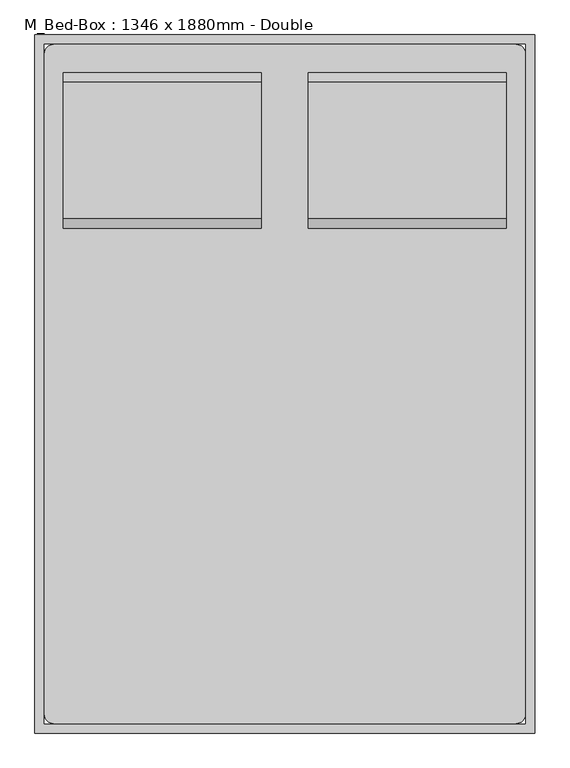
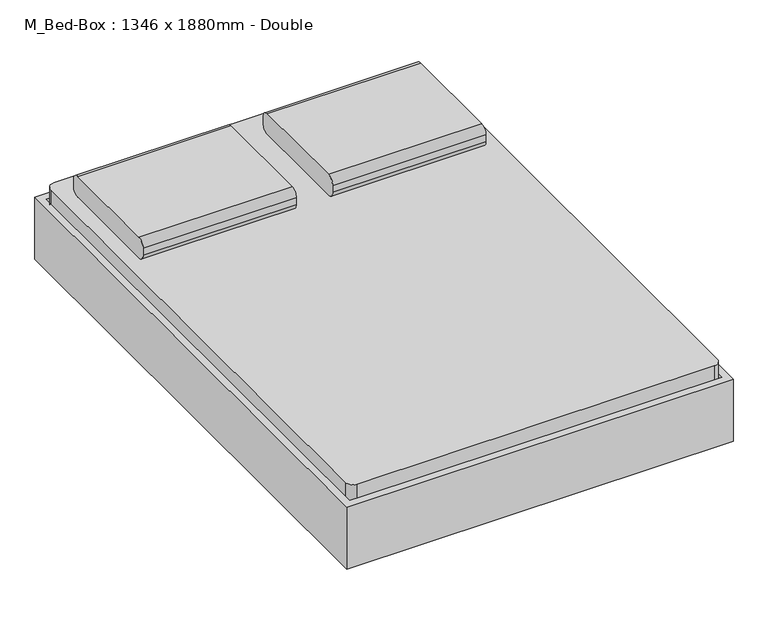
"""IFC4 building model written with IfcOpenShell, lengths in millimetres: furniture geometry, M_Bed-Box : 1346 x 1880mm - Double."""

from ifc_helpers import new_model, si_unit, point, frame, frame_2d, origin, place, context, project, spatial, polyline, circle_curve, trimmed, segment, composite_curve, outline, extrude, source, transform, mapped, element, save
from ifc_brep_helpers import plane_surface, cylinder_surface, revolved_surface, advanced_brep


def m_bed_box_1346_x_1880mm_double_b32eb57e(model_context):
    return source(origin(), model_context, "Body", "SolidModel", [
        extrude(outline(composite_curve([segment(polyline([(578.5704918, 406.4), (210.2704918, 406.4)]), True, "CONTINUOUS"), segment(trimmed(circle_curve(frame_2d((210.2704918, 431.8)), 25.4), [point((210.2704918, 406.4))], [point((184.8704918, 431.8))], False, "CARTESIAN"), True, "CONTINUOUS"), segment(polyline([(184.8704918, 431.8), (184.8704918, 457.2)]), True, "CONTINUOUS"), segment(trimmed(circle_curve(frame_2d((210.2704918, 457.2)), 25.4), [point((184.8704918, 457.2))], [point((210.2704918, 482.6))], False, "CARTESIAN"), True, "CONTINUOUS"), segment(polyline([(210.2704918, 482.6), (578.5704918, 482.6)]), True, "CONTINUOUS"), segment(trimmed(circle_curve(frame_2d((578.5704918, 457.2)), 25.4), [point((578.5704918, 482.6))], [point((603.9704918, 457.2))], False, "CARTESIAN"), True, "CONTINUOUS"), segment(polyline([(603.9704918, 457.2), (603.9704918, 431.8)]), True, "CONTINUOUS"), segment(trimmed(circle_curve(frame_2d((578.5704918, 431.8)), 25.4), [point((603.9704918, 431.8))], [point((578.5704918, 406.4))], False, "CARTESIAN"), True, "CONTINUOUS")], self_intersect=False)), frame((402.652459, 0.0, 0.0), z_axis=(1.0, 0.0, 0.0), x_axis=(0.0, 1.0, 0.0)), (0.0, 0.0, 1.0), 533.3),
        extrude(outline(composite_curve([segment(polyline([(578.5704918, 406.4), (210.2704918, 406.4)]), True, "CONTINUOUS"), segment(trimmed(circle_curve(frame_2d((210.2704918, 431.8)), 25.4), [point((210.2704918, 406.4))], [point((184.8704918, 431.8))], False, "CARTESIAN"), True, "CONTINUOUS"), segment(polyline([(184.8704918, 431.8), (184.8704918, 457.2)]), True, "CONTINUOUS"), segment(trimmed(circle_curve(frame_2d((210.2704918, 457.2)), 25.4), [point((184.8704918, 457.2))], [point((210.2704918, 482.6))], False, "CARTESIAN"), True, "CONTINUOUS"), segment(polyline([(210.2704918, 482.6), (578.5704918, 482.6)]), True, "CONTINUOUS"), segment(trimmed(circle_curve(frame_2d((578.5704918, 457.2)), 25.4), [point((578.5704918, 482.6))], [point((603.9704918, 457.2))], False, "CARTESIAN"), True, "CONTINUOUS"), segment(polyline([(603.9704918, 457.2), (603.9704918, 431.8)]), True, "CONTINUOUS"), segment(trimmed(circle_curve(frame_2d((578.5704918, 431.8)), 25.4), [point((603.9704918, 431.8))], [point((578.5704918, 406.4))], False, "CARTESIAN"), True, "CONTINUOUS")], self_intersect=False)), frame((-257.647541, 0.0, 0.0), z_axis=(1.0, 0.0, 0.0), x_axis=(0.0, 1.0, 0.0)), (0.0, 0.0, 1.0), 533.3),
        advanced_brep(
        [(-308.1231784, 451.5704918, 177.8), (-308.1231784, 375.3704918, 177.8), (-308.1231784, 375.3704918, 196.85), (-308.1231784, 451.5704918, 196.85), (-257.3231784, 451.5704918, 177.8), (-257.3231784, 375.3704918, 177.8), (-245.1869899, 375.3704918, 196.85), (-245.1869899, 451.5704918, 196.85), (-181.2523099, 451.5704918, 14.6654962), (-181.2523099, 375.3704918, 14.6654962), (-163.9871466, 375.3704918, 22.716374), (-163.9871466, 451.5704918, 22.716374), (-158.2320921, 375.3704918, 0.0), (-158.2320921, 451.5704918, 0.0), (-158.2320921, 375.3704918, 19.05), (-158.2320921, 451.5704918, 19.05), (-79.6195862, 451.5704918, 0.0), (-79.6195862, 375.3704918, 0.0), (-79.6195862, 375.3704918, 19.05), (-79.6195862, 451.5704918, 19.05), (-66.9195862, 375.3704918, 3.4029547), (-66.9195862, 451.5704918, 3.4029547), (-76.4445862, 375.3704918, 19.9007387), (-76.4445862, 451.5704918, 19.9007387), (-6.822541, 451.5704918, 38.1), (-6.822541, 375.3704918, 38.1), (-11.9269731, 375.3704918, 57.15), (-11.9269731, 451.5704918, 57.15), (685.4518216, 451.5704918, 38.1), (685.4518216, 375.3704918, 38.1), (690.5562537, 375.3704918, 57.15), (690.5562537, 451.5704918, 57.15), (745.5488669, 451.5704918, 3.4029547), (745.5488669, 375.3704918, 3.4029547), (755.0738669, 375.3704918, 19.9007387), (755.0738669, 451.5704918, 19.9007387), (758.2488669, 375.3704918, 0.0), (758.2488669, 451.5704918, 0.0), (758.2488669, 375.3704918, 19.05), (758.2488669, 451.5704918, 19.05), (836.8613728, 451.5704918, 0.0), (836.8613728, 375.3704918, 0.0), (836.8613728, 375.3704918, 19.05), (836.8613728, 451.5704918, 19.05), (859.8815906, 375.3704918, 14.6654962), (859.8815906, 451.5704918, 14.6654962), (842.6164272, 375.3704918, 22.716374), (842.6164272, 451.5704918, 22.716374), (935.952459, 451.5704918, 177.8), (935.952459, 375.3704918, 177.8), (923.8162705, 375.3704918, 196.85), (923.8162705, 451.5704918, 196.85), (986.752459, 451.5704918, 177.8), (986.752459, 451.5704918, 196.85), (986.752459, 375.3704918, 196.85), (986.752459, 375.3704918, 177.8)],
        [
            (0, 1),
            (1, 2),
            (2, 3),
            (3, 0),
            (0, 4),
            (4, 5),
            (5, 1),
            (5, 6),
            (6, 2),
            (6, 7),
            (7, 3),
            (7, 4),
            (4, 8),
            (8, 9),
            (9, 5),
            (9, 10),
            (10, 6),
            (10, 11),
            (11, 7),
            (11, 8),
            (12, 9, circle_curve(frame((-158.2320921, 375.3704918, 25.4), z_axis=(0.0, 1.0, 0.0), x_axis=(-0.906307787036649, 0.0, -0.4226182617407015)), 25.4)),
            (8, 13, circle_curve(frame((-158.2320921, 451.5704918, 25.4), z_axis=(0.0, -1.0, 0.0), x_axis=(-0.906307787036649, 0.0, -0.4226182617407015)), 25.4)),
            (13, 12),
            (14, 10, circle_curve(frame((-158.2320921, 375.3704918, 25.4), z_axis=(0.0, 1.0, 0.0), x_axis=(-0.906307787036649, 0.0, -0.4226182617407015)), 6.35)),
            (12, 14),
            (15, 11, circle_curve(frame((-158.2320921, 451.5704918, 25.4), z_axis=(0.0, 1.0, 0.0), x_axis=(-0.906307787036649, 0.0, -0.4226182617407015)), 6.35)),
            (14, 15),
            (15, 13),
            (13, 16),
            (16, 17),
            (17, 12),
            (17, 18),
            (18, 14),
            (18, 19),
            (19, 15),
            (19, 16),
            (20, 17, circle_curve(frame((-79.6195862, 375.3704918, 25.4), z_axis=(0.0, 1.0, 0.0), x_axis=(0.0, 0.0, -1.0)), 25.4)),
            (16, 21, circle_curve(frame((-79.6195862, 451.5704918, 25.4), z_axis=(0.0, -1.0, 0.0), x_axis=(0.0, 0.0, -1.0)), 25.4)),
            (21, 20),
            (22, 18, circle_curve(frame((-79.6195862, 375.3704918, 25.4), z_axis=(0.0, 1.0, 0.0), x_axis=(0.0, 0.0, -1.0)), 6.35)),
            (20, 22),
            (23, 19, circle_curve(frame((-79.6195862, 451.5704918, 25.4), z_axis=(0.0, 1.0, 0.0), x_axis=(0.0, 0.0, -1.0)), 6.35)),
            (22, 23),
            (23, 21),
            (21, 24),
            (24, 25),
            (25, 20),
            (25, 26),
            (26, 22),
            (26, 27),
            (27, 23),
            (27, 24),
            (24, 28),
            (28, 29),
            (29, 25),
            (29, 30),
            (30, 26),
            (30, 31),
            (31, 27),
            (31, 28),
            (28, 32),
            (32, 33),
            (33, 29),
            (33, 34),
            (34, 30),
            (34, 35),
            (35, 31),
            (35, 32),
            (36, 33, circle_curve(frame((758.2488669, 375.3704918, 25.4), z_axis=(0.0, 1.0, 0.0), x_axis=(-0.5000000000000463, 0.0, -0.8660254037844118)), 25.4)),
            (32, 37, circle_curve(frame((758.2488669, 451.5704918, 25.4), z_axis=(0.0, -1.0, 0.0), x_axis=(-0.5000000000000463, 0.0, -0.8660254037844118)), 25.4)),
            (37, 36),
            (38, 34, circle_curve(frame((758.2488669, 375.3704918, 25.4), z_axis=(0.0, 1.0, 0.0), x_axis=(-0.5000000000000463, 0.0, -0.8660254037844118)), 6.35)),
            (36, 38),
            (39, 35, circle_curve(frame((758.2488669, 451.5704918, 25.4), z_axis=(0.0, 1.0, 0.0), x_axis=(-0.5000000000000463, 0.0, -0.8660254037844118)), 6.35)),
            (38, 39),
            (39, 37),
            (37, 40),
            (40, 41),
            (41, 36),
            (41, 42),
            (42, 38),
            (42, 43),
            (43, 39),
            (43, 40),
            (44, 41, circle_curve(frame((836.8613728, 375.3704918, 25.4), z_axis=(0.0, 1.0, 0.0), x_axis=(0.0, 0.0, -1.0)), 25.4)),
            (40, 45, circle_curve(frame((836.8613728, 451.5704918, 25.4), z_axis=(0.0, -1.0, 0.0), x_axis=(0.0, 0.0, -1.0)), 25.4)),
            (45, 44),
            (46, 42, circle_curve(frame((836.8613728, 375.3704918, 25.4), z_axis=(0.0, 1.0, 0.0), x_axis=(0.0, 0.0, -1.0)), 6.35)),
            (44, 46),
            (47, 43, circle_curve(frame((836.8613728, 451.5704918, 25.4), z_axis=(0.0, 1.0, 0.0), x_axis=(0.0, 0.0, -1.0)), 6.35)),
            (46, 47),
            (47, 45),
            (45, 48),
            (48, 49),
            (49, 44),
            (49, 50),
            (50, 46),
            (50, 51),
            (51, 47),
            (51, 48),
            (52, 53),
            (53, 54),
            (54, 55),
            (55, 52),
            (48, 52),
            (55, 49),
            (54, 50),
            (53, 51),
        ],
        [
            plane_surface(frame((-308.1231784, 705.5704918, -152.9490627), z_axis=(-1.0, 0.0, 0.0), x_axis=(0.0, 1.0, 0.0))),
            plane_surface(frame((-308.1231784, 451.5704918, 177.8), z_axis=(0.0, 0.0, -1.0), x_axis=(1.0, 0.0, 0.0))),
            plane_surface(frame((-308.1231784, 375.3704918, 177.8), z_axis=(0.0, -1.0, 0.0), x_axis=(1.0, 0.0, 0.0))),
            plane_surface(frame((-308.1231784, 375.3704918, 196.85), z_axis=(0.0, 0.0, 1.0), x_axis=(1.0, 0.0, 0.0))),
            plane_surface(frame((-308.1231784, 451.5704918, 196.85), z_axis=(0.0, 1.0, 0.0), x_axis=(1.0, 0.0, 0.0))),
            plane_surface(frame((-257.3231784, 451.5704918, 177.8), z_axis=(-0.9063077870366486, 0.0, -0.4226182617407026), x_axis=(0.4226182617407026, 0.0, -0.9063077870366486))),
            plane_surface(frame((-257.3231784, 375.3704918, 177.8), z_axis=(0.0, -1.0000000000000002, 0.0), x_axis=(0.4226182617407026, 0.0, -0.9063077870366486))),
            plane_surface(frame((-245.1869899, 375.3704918, 196.85), z_axis=(0.9063077870366487, 0.0, 0.4226182617407023), x_axis=(0.4226182617407023, 0.0, -0.9063077870366487))),
            plane_surface(frame((-245.1869899, 451.5704918, 196.85), z_axis=(0.0, 1.0, 0.0), x_axis=(0.4226182617407027, 0.0, -0.9063077870366485))),
            cylinder_surface(frame((-158.2320921, 705.5704918, 25.4), z_axis=(0.0, -1.0, 0.0), x_axis=(-0.906307787036649, 0.0, -0.4226182617407015)), 25.4),
            plane_surface(frame((-158.2320921, 375.3704918, 25.4), z_axis=(0.0, -1.0, 0.0), x_axis=(-0.906307787036649, 0.0, -0.4226182617407015))),
            revolved_surface(polyline([(-163.9871465476827, 375.3704918, 22.716374037946544), (-163.9871465476827, 451.5704918, 22.716374037946544)]), (-158.2320921, 705.5704918, 25.4), (0.0, -1.0, 0.0)),
            plane_surface(frame((-158.2320921, 451.5704918, 25.4), z_axis=(0.0, 1.0, 0.0), x_axis=(-0.906307787036649, 0.0, -0.4226182617407015))),
            plane_surface(frame((-158.2320921, 451.5704918, 0.0), z_axis=(0.0, 0.0, -1.0), x_axis=(1.0, 0.0, 0.0))),
            plane_surface(frame((-158.2320921, 375.3704918, 0.0), z_axis=(0.0, -1.0, 0.0), x_axis=(1.0, 0.0, 0.0))),
            plane_surface(frame((-158.2320921, 375.3704918, 19.05), z_axis=(0.0, 0.0, 1.0), x_axis=(1.0, 0.0, 0.0))),
            plane_surface(frame((-158.2320921, 451.5704918, 19.05), z_axis=(0.0, 1.0, 0.0), x_axis=(1.0, 0.0, 0.0))),
            cylinder_surface(frame((-79.6195862, 705.5704918, 25.4), z_axis=(0.0, -1.0, 0.0), x_axis=(0.0, 0.0, -1.0)), 25.4),
            plane_surface(frame((-79.6195862, 375.3704918, 25.4), z_axis=(0.0, -1.0, 0.0), x_axis=(0.0, 0.0, -1.0))),
            revolved_surface(polyline([(-79.6195862, 375.3704918, 19.049999999999997), (-79.6195862, 451.5704918, 19.049999999999997)]), (-79.6195862, 705.5704918, 25.4), (0.0, -1.0, 0.0)),
            plane_surface(frame((-79.6195862, 451.5704918, 25.4), z_axis=(0.0, 1.0, 0.0), x_axis=(0.0, 0.0, -1.0))),
            plane_surface(frame((-66.9195862, 451.5704918, 3.4029547), z_axis=(0.4999999999998744, 0.0, -0.8660254037845112), x_axis=(0.8660254037845112, 0.0, 0.4999999999998744))),
            plane_surface(frame((-66.9195862, 375.3704918, 3.4029547), z_axis=(0.0, -1.0000000000000002, 0.0), x_axis=(0.8660254037845112, 0.0, 0.4999999999998745))),
            plane_surface(frame((-76.4445862, 375.3704918, 19.9007387), z_axis=(-0.4999999999998741, 0.0, 0.8660254037845113), x_axis=(0.8660254037845113, 0.0, 0.4999999999998741))),
            plane_surface(frame((-76.4445862, 451.5704918, 19.9007387), z_axis=(0.0, 1.0, 0.0), x_axis=(0.866025403784511, 0.0, 0.49999999999987477))),
            plane_surface(frame((-6.822541, 451.5704918, 38.1), z_axis=(0.0, 0.0, -1.0), x_axis=(1.0, 0.0, 0.0))),
            plane_surface(frame((-6.822541, 375.3704918, 38.1), z_axis=(0.0, -1.0, 0.0), x_axis=(1.0, 0.0, 0.0))),
            plane_surface(frame((-11.9269731, 375.3704918, 57.15), z_axis=(0.0, 0.0, 1.0), x_axis=(1.0, 0.0, 0.0))),
            plane_surface(frame((-11.9269731, 451.5704918, 57.15), z_axis=(0.0, 1.0, 0.0), x_axis=(1.0, 0.0, 0.0))),
            plane_surface(frame((685.4518216, 451.5704918, 38.1), z_axis=(-0.5000000000000494, 0.0, -0.8660254037844102), x_axis=(0.8660254037844102, 0.0, -0.5000000000000494))),
            plane_surface(frame((685.4518216, 375.3704918, 38.1), z_axis=(0.0, -1.0, 0.0), x_axis=(0.8660254037844112, 0.0, -0.5000000000000476))),
            plane_surface(frame((690.5562537, 375.3704918, 57.15), z_axis=(0.5000000000000488, 0.0, 0.8660254037844105), x_axis=(0.8660254037844105, 0.0, -0.5000000000000488))),
            plane_surface(frame((690.5562537, 451.5704918, 57.15), z_axis=(0.0, 1.0, 0.0), x_axis=(0.8660254037844106, 0.0, -0.5000000000000485))),
            cylinder_surface(frame((758.2488669, 705.5704918, 25.4), z_axis=(0.0, -1.0, 0.0), x_axis=(-0.5000000000000463, 0.0, -0.8660254037844118)), 25.4),
            plane_surface(frame((758.2488669, 375.3704918, 25.4), z_axis=(0.0, -1.0000000000000002, 0.0), x_axis=(-0.5000000000000464, 0.0, -0.866025403784412))),
            revolved_surface(polyline([(755.0738668999998, 375.3704918, 19.90073868596898), (755.0738668999998, 451.5704918, 19.90073868596898)]), (758.2488669, 705.5704918, 25.4), (0.0, -1.0, 0.0)),
            plane_surface(frame((758.2488669, 451.5704918, 25.4), z_axis=(0.0, 1.0000000000000002, 0.0), x_axis=(-0.5000000000000464, 0.0, -0.866025403784412))),
            plane_surface(frame((758.2488669, 451.5704918, 0.0), z_axis=(0.0, 0.0, -1.0), x_axis=(1.0, 0.0, 0.0))),
            plane_surface(frame((758.2488669, 375.3704918, 0.0), z_axis=(0.0, -1.0, 0.0), x_axis=(1.0, 0.0, 0.0))),
            plane_surface(frame((758.2488669, 375.3704918, 19.05), z_axis=(0.0, 0.0, 1.0), x_axis=(1.0, 0.0, 0.0))),
            plane_surface(frame((758.2488669, 451.5704918, 19.05), z_axis=(0.0, 1.0, 0.0), x_axis=(1.0, 0.0, 0.0))),
            cylinder_surface(frame((836.8613728, 705.5704918, 25.4), z_axis=(0.0, -1.0, 0.0), x_axis=(0.0, 0.0, -1.0)), 25.4),
            plane_surface(frame((836.8613728, 375.3704918, 25.4), z_axis=(0.0, -1.0, 0.0), x_axis=(0.0, 0.0, -1.0))),
            revolved_surface(polyline([(836.8613728, 375.3704918, 19.049999999999997), (836.8613728, 451.5704918, 19.049999999999997)]), (836.8613728, 705.5704918, 25.4), (0.0, -1.0, 0.0)),
            plane_surface(frame((836.8613728, 451.5704918, 25.4), z_axis=(0.0, 1.0, 0.0), x_axis=(0.0, 0.0, -1.0))),
            plane_surface(frame((859.8815906, 451.5704918, 14.6654962), z_axis=(0.90630778703668, 0.0, -0.422618261740635), x_axis=(0.422618261740635, 0.0, 0.90630778703668))),
            plane_surface(frame((859.8815906, 375.3704918, 14.6654962), z_axis=(0.0, -1.0000000000000002, 0.0), x_axis=(0.4226182617406349, 0.0, 0.9063077870366801))),
            plane_surface(frame((842.6164272, 375.3704918, 22.716374), z_axis=(-0.9063077870366805, 0.0, 0.4226182617406341), x_axis=(0.4226182617406341, 0.0, 0.9063077870366805))),
            plane_surface(frame((842.6164272, 451.5704918, 22.716374), z_axis=(0.0, 1.0, 0.0), x_axis=(0.42261826174063455, 0.0, 0.9063077870366802))),
            plane_surface(frame((986.752459, 705.5704918, -152.9490627), z_axis=(1.0, 0.0, 0.0), x_axis=(0.0, 1.0, 0.0))),
            plane_surface(frame((935.952459, 451.5704918, 177.8), z_axis=(0.0, 0.0, -1.0), x_axis=(1.0, 0.0, 0.0))),
            plane_surface(frame((935.952459, 375.3704918, 177.8), z_axis=(0.0, -1.0, 0.0), x_axis=(1.0, 0.0, 0.0))),
            plane_surface(frame((923.8162705, 375.3704918, 196.85), z_axis=(0.0, 0.0, 1.0), x_axis=(1.0, 0.0, 0.0))),
            plane_surface(frame((923.8162705, 451.5704918, 196.85), z_axis=(0.0, 1.0, 0.0), x_axis=(1.0, 0.0, 0.0))),
        ],
        [
            (0, [[1, 2, 3, 4]]),
            (1, [[-1, 5, 6, 7]]),
            (2, [[-2, -7, 8, 9]]),
            (3, [[-3, -9, 10, 11]]),
            (4, [[-4, -11, 12, -5]]),
            (5, [[-6, 13, 14, 15]]),
            (6, [[-8, -15, 16, 17]]),
            (7, [[-10, -17, 18, 19]]),
            (8, [[-12, -19, 20, -13]]),
            (9, [[21, -14, 22, 23]]),
            (10, [[24, -16, -21, 25]]),
            (11, [[26, -18, -24, 27]]),
            (12, [[-22, -20, -26, 28]]),
            (13, [[-23, 29, 30, 31]]),
            (14, [[-25, -31, 32, 33]]),
            (15, [[-27, -33, 34, 35]]),
            (16, [[-28, -35, 36, -29]]),
            (17, [[37, -30, 38, 39]]),
            (18, [[40, -32, -37, 41]]),
            (19, [[42, -34, -40, 43]]),
            (20, [[-38, -36, -42, 44]]),
            (21, [[-39, 45, 46, 47]]),
            (22, [[-41, -47, 48, 49]]),
            (23, [[-43, -49, 50, 51]]),
            (24, [[-44, -51, 52, -45]]),
            (25, [[-46, 53, 54, 55]]),
            (26, [[-48, -55, 56, 57]]),
            (27, [[-50, -57, 58, 59]]),
            (28, [[-52, -59, 60, -53]]),
            (29, [[-54, 61, 62, 63]]),
            (30, [[-56, -63, 64, 65]]),
            (31, [[-58, -65, 66, 67]]),
            (32, [[-60, -67, 68, -61]]),
            (33, [[69, -62, 70, 71]]),
            (34, [[72, -64, -69, 73]]),
            (35, [[74, -66, -72, 75]]),
            (36, [[-70, -68, -74, 76]]),
            (37, [[-71, 77, 78, 79]]),
            (38, [[-73, -79, 80, 81]]),
            (39, [[-75, -81, 82, 83]]),
            (40, [[-76, -83, 84, -77]]),
            (41, [[85, -78, 86, 87]]),
            (42, [[88, -80, -85, 89]]),
            (43, [[90, -82, -88, 91]]),
            (44, [[-86, -84, -90, 92]]),
            (45, [[-87, 93, 94, 95]]),
            (46, [[-89, -95, 96, 97]]),
            (47, [[-91, -97, 98, 99]]),
            (48, [[-92, -99, 100, -93]]),
            (49, [[101, 102, 103, 104]]),
            (50, [[-94, 105, -104, 106]]),
            (51, [[-96, -106, -103, 107]]),
            (52, [[-98, -107, -102, 108]]),
            (53, [[-100, -108, -101, -105]]),
        ],
    ),
        extrude(outline(composite_curve([segment(polyline([(-283.047541, 680.1704918), (961.352459, 680.1704918)]), True, "CONTINUOUS"), segment(trimmed(circle_curve(frame_2d((961.352459, 654.7704918)), 25.4), [point((961.352459, 680.1704918))], [point((986.752459, 654.7704918))], False, "CARTESIAN"), True, "CONTINUOUS"), segment(polyline([(986.752459, 654.7704918), (986.752459, -1123.6295082)]), True, "CONTINUOUS"), segment(trimmed(circle_curve(frame_2d((961.352459, -1123.6295082)), 25.4), [point((986.752459, -1123.6295082))], [point((961.352459, -1149.0295082))], False, "CARTESIAN"), True, "CONTINUOUS"), segment(polyline([(961.352459, -1149.0295082), (-283.047541, -1149.0295082)]), True, "CONTINUOUS"), segment(trimmed(circle_curve(frame_2d((-283.047541, -1123.6295082)), 25.4), [point((-283.047541, -1149.0295082))], [point((-308.447541, -1123.6295082))], False, "CARTESIAN"), True, "CONTINUOUS"), segment(polyline([(-308.447541, -1123.6295082), (-308.447541, 654.7704918)]), True, "CONTINUOUS"), segment(trimmed(circle_curve(frame_2d((-283.047541, 654.7704918)), 25.4), [point((-308.447541, 654.7704918))], [point((-283.047541, 680.1704918))], False, "CARTESIAN"), True, "CONTINUOUS")], self_intersect=False)), frame((0.0, 0.0, 203.2), z_axis=(0.0, 0.0, 1.0), x_axis=(1.0, 0.0, 0.0)), (0.0, 0.0, 1.0), 203.2),
        advanced_brep(
        [(-308.447541, -869.6295082, 196.85), (-308.447541, -869.6295082, 177.8), (-308.447541, -945.8295082, 177.8), (-308.447541, -945.8295082, 196.85), (-245.5113525, -869.6295082, 196.85), (-257.647541, -869.6295082, 177.8), (-257.647541, -945.8295082, 177.8), (-245.5113525, -945.8295082, 196.85), (-164.3115092, -869.6295082, 22.716374), (-181.5766725, -869.6295082, 14.6654962), (-181.5766725, -945.8295082, 14.6654962), (-164.3115092, -945.8295082, 22.716374), (-158.5564547, -869.6295082, 0.0), (-158.5564547, -869.6295082, 19.05), (-158.5564547, -945.8295082, 0.0), (-158.5564547, -945.8295082, 19.05), (-79.9439489, -869.6295082, 19.05), (-79.9439489, -869.6295082, 0.0), (-79.9439489, -945.8295082, 0.0), (-79.9439489, -945.8295082, 19.05), (-67.2439489, -869.6295082, 3.4029547), (-76.7689489, -869.6295082, 19.9007387), (-67.2439489, -945.8295082, 3.4029547), (-76.7689489, -945.8295082, 19.9007387), (-12.2513357, -869.6295082, 57.15), (-7.1469036, -869.6295082, 38.1), (-7.1469036, -945.8295082, 38.1), (-12.2513357, -945.8295082, 57.15), (690.5562537, -869.6295082, 57.15), (685.4518216, -869.6295082, 38.1), (685.4518216, -945.8295082, 38.1), (690.5562537, -945.8295082, 57.15), (755.0738669, -869.6295082, 19.9007387), (745.5488669, -869.6295082, 3.4029547), (745.5488669, -945.8295082, 3.4029547), (755.0738669, -945.8295082, 19.9007387), (758.2488669, -869.6295082, 0.0), (758.2488669, -869.6295082, 19.05), (758.2488669, -945.8295082, 0.0), (758.2488669, -945.8295082, 19.05), (836.8613728, -869.6295082, 19.05), (836.8613728, -869.6295082, 0.0), (836.8613728, -945.8295082, 0.0), (836.8613728, -945.8295082, 19.05), (859.8815906, -869.6295082, 14.6654962), (842.6164272, -869.6295082, 22.716374), (859.8815906, -945.8295082, 14.6654962), (842.6164272, -945.8295082, 22.716374), (923.8162705, -869.6295082, 196.85), (935.952459, -869.6295082, 177.8), (935.952459, -945.8295082, 177.8), (923.8162705, -945.8295082, 196.85), (986.752459, -869.6295082, 196.85), (986.752459, -945.8295082, 196.85), (986.752459, -945.8295082, 177.8), (986.752459, -869.6295082, 177.8)],
        [
            (0, 1),
            (1, 2),
            (2, 3),
            (3, 0),
            (0, 4),
            (4, 5),
            (5, 1),
            (5, 6),
            (6, 2),
            (6, 7),
            (7, 3),
            (7, 4),
            (4, 8),
            (8, 9),
            (9, 5),
            (9, 10),
            (10, 6),
            (10, 11),
            (11, 7),
            (11, 8),
            (12, 9, circle_curve(frame((-158.5564547, -869.6295082, 25.4), z_axis=(0.0, 1.0, 0.0), x_axis=(-0.9063077870366625, 0.0, -0.4226182617406725)), 25.4)),
            (8, 13, circle_curve(frame((-158.5564547, -869.6295082, 25.4), z_axis=(0.0, -1.0, 0.0), x_axis=(-0.9063077870366625, 0.0, -0.4226182617406725)), 6.35)),
            (13, 12),
            (14, 10, circle_curve(frame((-158.5564547, -945.8295082, 25.4), z_axis=(0.0, 1.0, 0.0), x_axis=(-0.9063077870366625, 0.0, -0.4226182617406725)), 25.4)),
            (12, 14),
            (15, 11, circle_curve(frame((-158.5564547, -945.8295082, 25.4), z_axis=(0.0, 1.0, 0.0), x_axis=(-0.9063077870366625, 0.0, -0.4226182617406725)), 6.35)),
            (14, 15),
            (15, 13),
            (13, 16),
            (16, 17),
            (17, 12),
            (17, 18),
            (18, 14),
            (18, 19),
            (19, 15),
            (19, 16),
            (20, 17, circle_curve(frame((-79.9439489, -869.6295082, 25.4), z_axis=(0.0, 1.0, 0.0), x_axis=(0.0, 0.0, -1.0)), 25.4)),
            (16, 21, circle_curve(frame((-79.9439489, -869.6295082, 25.4), z_axis=(0.0, -1.0, 0.0), x_axis=(0.0, 0.0, -1.0)), 6.35)),
            (21, 20),
            (22, 18, circle_curve(frame((-79.9439489, -945.8295082, 25.4), z_axis=(0.0, 1.0, 0.0), x_axis=(0.0, 0.0, -1.0)), 25.4)),
            (20, 22),
            (23, 19, circle_curve(frame((-79.9439489, -945.8295082, 25.4), z_axis=(0.0, 1.0, 0.0), x_axis=(0.0, 0.0, -1.0)), 6.35)),
            (22, 23),
            (23, 21),
            (21, 24),
            (24, 25),
            (25, 20),
            (25, 26),
            (26, 22),
            (26, 27),
            (27, 23),
            (27, 24),
            (24, 28),
            (28, 29),
            (29, 25),
            (29, 30),
            (30, 26),
            (30, 31),
            (31, 27),
            (31, 28),
            (28, 32),
            (32, 33),
            (33, 29),
            (33, 34),
            (34, 30),
            (34, 35),
            (35, 31),
            (35, 32),
            (36, 33, circle_curve(frame((758.2488669, -869.6295082, 25.4), z_axis=(0.0, 1.0, 0.0), x_axis=(-0.5000000000000528, 0.0, -0.8660254037844081)), 25.4)),
            (32, 37, circle_curve(frame((758.2488669, -869.6295082, 25.4), z_axis=(0.0, -1.0, 0.0), x_axis=(-0.5000000000000528, 0.0, -0.8660254037844081)), 6.35)),
            (37, 36),
            (38, 34, circle_curve(frame((758.2488669, -945.8295082, 25.4), z_axis=(0.0, 1.0, 0.0), x_axis=(-0.5000000000000528, 0.0, -0.8660254037844081)), 25.4)),
            (36, 38),
            (39, 35, circle_curve(frame((758.2488669, -945.8295082, 25.4), z_axis=(0.0, 1.0, 0.0), x_axis=(-0.5000000000000528, 0.0, -0.8660254037844081)), 6.35)),
            (38, 39),
            (39, 37),
            (37, 40),
            (40, 41),
            (41, 36),
            (41, 42),
            (42, 38),
            (42, 43),
            (43, 39),
            (43, 40),
            (44, 41, circle_curve(frame((836.8613728, -869.6295082, 25.4), z_axis=(0.0, 1.0, 0.0), x_axis=(0.0, 0.0, -1.0)), 25.4)),
            (40, 45, circle_curve(frame((836.8613728, -869.6295082, 25.4), z_axis=(0.0, -1.0, 0.0), x_axis=(0.0, 0.0, -1.0)), 6.35)),
            (45, 44),
            (46, 42, circle_curve(frame((836.8613728, -945.8295082, 25.4), z_axis=(0.0, 1.0, 0.0), x_axis=(0.0, 0.0, -1.0)), 25.4)),
            (44, 46),
            (47, 43, circle_curve(frame((836.8613728, -945.8295082, 25.4), z_axis=(0.0, 1.0, 0.0), x_axis=(0.0, 0.0, -1.0)), 6.35)),
            (46, 47),
            (47, 45),
            (45, 48),
            (48, 49),
            (49, 44),
            (49, 50),
            (50, 46),
            (50, 51),
            (51, 47),
            (51, 48),
            (52, 53),
            (53, 54),
            (54, 55),
            (55, 52),
            (48, 52),
            (55, 49),
            (54, 50),
            (53, 51),
        ],
        [
            plane_surface(frame((-308.447541, -1174.4295082, -127.5947323), z_axis=(-1.0, 0.0, 0.0), x_axis=(0.0, 1.0, 0.0))),
            plane_surface(frame((-308.447541, -869.6295082, 196.85), z_axis=(0.0, 1.0, 0.0), x_axis=(1.0, 0.0, 0.0))),
            plane_surface(frame((-308.447541, -869.6295082, 177.8), z_axis=(0.0, 0.0, -1.0), x_axis=(1.0, 0.0, 0.0))),
            plane_surface(frame((-308.447541, -945.8295082, 177.8), z_axis=(0.0, -1.0, 0.0), x_axis=(1.0, 0.0, 0.0))),
            plane_surface(frame((-308.447541, -945.8295082, 196.85), z_axis=(0.0, 0.0, 1.0), x_axis=(1.0, 0.0, 0.0))),
            plane_surface(frame((-245.5113525, -869.6295082, 196.85), z_axis=(0.0, 1.0, 0.0), x_axis=(0.4226182617406714, 0.0, -0.906307787036663))),
            plane_surface(frame((-257.647541, -869.6295082, 177.8), z_axis=(-0.9063077870366631, 0.0, -0.42261826174067146), x_axis=(0.42261826174067146, 0.0, -0.9063077870366631))),
            plane_surface(frame((-257.647541, -945.8295082, 177.8), z_axis=(0.0, -1.0000000000000002, 0.0), x_axis=(0.4226182617406716, 0.0, -0.906307787036663))),
            plane_surface(frame((-245.5113525, -945.8295082, 196.85), z_axis=(0.906307787036663, 0.0, 0.4226182617406716), x_axis=(0.4226182617406716, 0.0, -0.906307787036663))),
            plane_surface(frame((-158.5564547, -869.6295082, 25.4), z_axis=(0.0, 1.0, 0.0), x_axis=(-0.9063077870366625, 0.0, -0.4226182617406725))),
            cylinder_surface(frame((-158.5564547, -1174.4295082, 25.4), z_axis=(0.0, -1.0, 0.0), x_axis=(-0.9063077870366625, 0.0, -0.4226182617406725)), 25.4),
            plane_surface(frame((-158.5564547, -945.8295082, 25.4), z_axis=(0.0, -1.0, 0.0), x_axis=(-0.9063077870366625, 0.0, -0.4226182617406725))),
            revolved_surface(polyline([(-164.31150914768278, -945.8295082, 22.71637403794673), (-164.31150914768278, -869.6295082, 22.71637403794673)]), (-158.5564547, -1174.4295082, 25.4), (0.0, -1.0, 0.0)),
            plane_surface(frame((-158.5564547, -869.6295082, 19.05), z_axis=(0.0, 1.0, 0.0), x_axis=(1.0, 0.0, 0.0))),
            plane_surface(frame((-158.5564547, -869.6295082, 0.0), z_axis=(0.0, 0.0, -1.0), x_axis=(1.0, 0.0, 0.0))),
            plane_surface(frame((-158.5564547, -945.8295082, 0.0), z_axis=(0.0, -1.0, 0.0), x_axis=(1.0, 0.0, 0.0))),
            plane_surface(frame((-158.5564547, -945.8295082, 19.05), z_axis=(0.0, 0.0, 1.0), x_axis=(1.0, 0.0, 0.0))),
            plane_surface(frame((-79.9439489, -869.6295082, 25.4), z_axis=(0.0, 1.0, 0.0), x_axis=(0.0, 0.0, -1.0))),
            cylinder_surface(frame((-79.9439489, -1174.4295082, 25.4), z_axis=(0.0, -1.0, 0.0), x_axis=(0.0, 0.0, -1.0)), 25.4),
            plane_surface(frame((-79.9439489, -945.8295082, 25.4), z_axis=(0.0, -1.0, 0.0), x_axis=(0.0, 0.0, -1.0))),
            revolved_surface(polyline([(-79.9439489, -945.8295082, 19.049999999999997), (-79.9439489, -869.6295082, 19.049999999999997)]), (-79.9439489, -1174.4295082, 25.4), (0.0, -1.0, 0.0)),
            plane_surface(frame((-76.7689489, -869.6295082, 19.9007387), z_axis=(0.0, 1.0000000000000002, 0.0), x_axis=(0.8660254037844788, 0.0, 0.49999999999993067))),
            plane_surface(frame((-67.2439489, -869.6295082, 3.4029547), z_axis=(0.49999999999993067, 0.0, -0.8660254037844787), x_axis=(0.8660254037844787, 0.0, 0.49999999999993067))),
            plane_surface(frame((-67.2439489, -945.8295082, 3.4029547), z_axis=(0.0, -1.0, 0.0), x_axis=(0.8660254037844782, 0.0, 0.4999999999999315))),
            plane_surface(frame((-76.7689489, -945.8295082, 19.9007387), z_axis=(-0.49999999999993044, 0.0, 0.8660254037844789), x_axis=(0.8660254037844789, 0.0, 0.49999999999993044))),
            plane_surface(frame((-12.2513357, -869.6295082, 57.15), z_axis=(0.0, 1.0, 0.0), x_axis=(1.0, 0.0, 0.0))),
            plane_surface(frame((-7.1469036, -869.6295082, 38.1), z_axis=(0.0, 0.0, -1.0), x_axis=(1.0, 0.0, 0.0))),
            plane_surface(frame((-7.1469036, -945.8295082, 38.1), z_axis=(0.0, -1.0, 0.0), x_axis=(1.0, 0.0, 0.0))),
            plane_surface(frame((-12.2513357, -945.8295082, 57.15), z_axis=(0.0, 0.0, 1.0), x_axis=(1.0, 0.0, 0.0))),
            plane_surface(frame((690.5562537, -869.6295082, 57.15), z_axis=(0.0, 1.0, 0.0), x_axis=(0.8660254037844087, 0.0, -0.5000000000000518))),
            plane_surface(frame((685.4518216, -869.6295082, 38.1), z_axis=(-0.5000000000000513, 0.0, -0.8660254037844092), x_axis=(0.8660254037844092, 0.0, -0.5000000000000513))),
            plane_surface(frame((685.4518216, -945.8295082, 38.1), z_axis=(0.0, -1.0, 0.0), x_axis=(0.8660254037844081, 0.0, -0.5000000000000531))),
            plane_surface(frame((690.5562537, -945.8295082, 57.15), z_axis=(0.5000000000000521, 0.0, 0.8660254037844086), x_axis=(0.8660254037844086, 0.0, -0.5000000000000521))),
            plane_surface(frame((758.2488669, -869.6295082, 25.4), z_axis=(0.0, 1.0000000000000002, 0.0), x_axis=(-0.500000000000053, 0.0, -0.8660254037844082))),
            cylinder_surface(frame((758.2488669, -1174.4295082, 25.4), z_axis=(0.0, -1.0, 0.0), x_axis=(-0.5000000000000528, 0.0, -0.8660254037844081)), 25.4),
            plane_surface(frame((758.2488669, -945.8295082, 25.4), z_axis=(0.0, -1.0000000000000002, 0.0), x_axis=(-0.500000000000053, 0.0, -0.8660254037844082))),
            revolved_surface(polyline([(755.0738668999998, -945.8295082, 19.900738685969007), (755.0738668999998, -869.6295082, 19.900738685969007)]), (758.2488669, -1174.4295082, 25.4), (0.0, -1.0, 0.0)),
            plane_surface(frame((758.2488669, -869.6295082, 19.05), z_axis=(0.0, 1.0, 0.0), x_axis=(1.0, 0.0, 0.0))),
            plane_surface(frame((758.2488669, -869.6295082, 0.0), z_axis=(0.0, 0.0, -1.0), x_axis=(1.0, 0.0, 0.0))),
            plane_surface(frame((758.2488669, -945.8295082, 0.0), z_axis=(0.0, -1.0, 0.0), x_axis=(1.0, 0.0, 0.0))),
            plane_surface(frame((758.2488669, -945.8295082, 19.05), z_axis=(0.0, 0.0, 1.0), x_axis=(1.0, 0.0, 0.0))),
            plane_surface(frame((836.8613728, -869.6295082, 25.4), z_axis=(0.0, 1.0, 0.0), x_axis=(0.0, 0.0, -1.0))),
            cylinder_surface(frame((836.8613728, -1174.4295082, 25.4), z_axis=(0.0, -1.0, 0.0), x_axis=(0.0, 0.0, -1.0)), 25.4),
            plane_surface(frame((836.8613728, -945.8295082, 25.4), z_axis=(0.0, -1.0, 0.0), x_axis=(0.0, 0.0, -1.0))),
            revolved_surface(polyline([(836.8613728, -945.8295082, 19.049999999999997), (836.8613728, -869.6295082, 19.049999999999997)]), (836.8613728, -1174.4295082, 25.4), (0.0, -1.0, 0.0)),
            plane_surface(frame((842.6164272, -869.6295082, 22.716374), z_axis=(0.0, 1.0, 0.0), x_axis=(0.4226182617405387, 0.0, 0.906307787036725))),
            plane_surface(frame((859.8815906, -869.6295082, 14.6654962), z_axis=(0.906307787036725, 0.0, -0.4226182617405386), x_axis=(0.4226182617405386, 0.0, 0.906307787036725))),
            plane_surface(frame((859.8815906, -945.8295082, 14.6654962), z_axis=(0.0, -1.0, 0.0), x_axis=(0.4226182617405387, 0.0, 0.906307787036725))),
            plane_surface(frame((842.6164272, -945.8295082, 22.716374), z_axis=(-0.9063077870367251, 0.0, 0.4226182617405384), x_axis=(0.4226182617405384, 0.0, 0.9063077870367251))),
            plane_surface(frame((986.752459, -1174.4295082, -127.5947323), z_axis=(1.0, 0.0, 0.0), x_axis=(0.0, 1.0, 0.0))),
            plane_surface(frame((923.8162705, -869.6295082, 196.85), z_axis=(0.0, 1.0, 0.0), x_axis=(1.0, 0.0, 0.0))),
            plane_surface(frame((935.952459, -869.6295082, 177.8), z_axis=(0.0, 0.0, -1.0), x_axis=(1.0, 0.0, 0.0))),
            plane_surface(frame((935.952459, -945.8295082, 177.8), z_axis=(0.0, -1.0, 0.0), x_axis=(1.0, 0.0, 0.0))),
            plane_surface(frame((923.8162705, -945.8295082, 196.85), z_axis=(0.0, 0.0, 1.0), x_axis=(1.0, 0.0, 0.0))),
        ],
        [
            (0, [[1, 2, 3, 4]]),
            (1, [[-1, 5, 6, 7]]),
            (2, [[-2, -7, 8, 9]]),
            (3, [[-3, -9, 10, 11]]),
            (4, [[-4, -11, 12, -5]]),
            (5, [[-6, 13, 14, 15]]),
            (6, [[-8, -15, 16, 17]]),
            (7, [[-10, -17, 18, 19]]),
            (8, [[-12, -19, 20, -13]]),
            (9, [[21, -14, 22, 23]]),
            (10, [[24, -16, -21, 25]]),
            (11, [[26, -18, -24, 27]]),
            (12, [[-22, -20, -26, 28]]),
            (13, [[-23, 29, 30, 31]]),
            (14, [[-25, -31, 32, 33]]),
            (15, [[-27, -33, 34, 35]]),
            (16, [[-28, -35, 36, -29]]),
            (17, [[37, -30, 38, 39]]),
            (18, [[40, -32, -37, 41]]),
            (19, [[42, -34, -40, 43]]),
            (20, [[-38, -36, -42, 44]]),
            (21, [[-39, 45, 46, 47]]),
            (22, [[-41, -47, 48, 49]]),
            (23, [[-43, -49, 50, 51]]),
            (24, [[-44, -51, 52, -45]]),
            (25, [[-46, 53, 54, 55]]),
            (26, [[-48, -55, 56, 57]]),
            (27, [[-50, -57, 58, 59]]),
            (28, [[-52, -59, 60, -53]]),
            (29, [[-54, 61, 62, 63]]),
            (30, [[-56, -63, 64, 65]]),
            (31, [[-58, -65, 66, 67]]),
            (32, [[-60, -67, 68, -61]]),
            (33, [[69, -62, 70, 71]]),
            (34, [[72, -64, -69, 73]]),
            (35, [[74, -66, -72, 75]]),
            (36, [[-70, -68, -74, 76]]),
            (37, [[-71, 77, 78, 79]]),
            (38, [[-73, -79, 80, 81]]),
            (39, [[-75, -81, 82, 83]]),
            (40, [[-76, -83, 84, -77]]),
            (41, [[85, -78, 86, 87]]),
            (42, [[88, -80, -85, 89]]),
            (43, [[90, -82, -88, 91]]),
            (44, [[-86, -84, -90, 92]]),
            (45, [[-87, 93, 94, 95]]),
            (46, [[-89, -95, 96, 97]]),
            (47, [[-91, -97, 98, 99]]),
            (48, [[-92, -99, 100, -93]]),
            (49, [[101, 102, 103, 104]]),
            (50, [[-94, 105, -104, 106]]),
            (51, [[-96, -106, -103, 107]]),
            (52, [[-98, -107, -102, 108]]),
            (53, [[-100, -108, -101, -105]]),
        ],
    ),
        extrude(outline(polyline([(1012.152459, 705.5704918), (1012.152459, -1174.4295082), (-333.847541, -1174.4295082), (-333.847541, 705.5704918), (1012.152459, 705.5704918)]), holes=[polyline([(986.752459, 680.1704918), (-308.447541, 680.1704918), (-308.447541, -1149.0295082), (986.752459, -1149.0295082), (986.752459, 680.1704918)])]), frame((0.0, 0.0, 127.0), z_axis=(0.0, 0.0, 1.0), x_axis=(1.0, 0.0, 0.0)), (0.0, 0.0, 1.0), 228.6),
    ])


if __name__ == "__main__":
    model = new_model("IFC4")
    model_context = context("Model", 3, world=origin())
    ifc_project = project(units=[si_unit("LENGTHUNIT", "METRE", prefix="MILLI")], contexts=[model_context])
    site = spatial("IfcSite", under=ifc_project)
    building = spatial("IfcBuilding", under=site)
    placement = place(None, origin())
    m_bed_box_1346_x_1880mm_double_shape = m_bed_box_1346_x_1880mm_double_b32eb57e(model_context)
    element("IfcFurniture", 1, ObjectType="M_Bed-Box : 1346 x 1880mm - Double", at=placement, inside=building, context=model_context, shape_type="MappedRepresentation", body=[
        mapped(m_bed_box_1346_x_1880mm_double_shape, transform((0.0, 0.0, 0.0), x_axis=(1.0, 0.0, 0.0), y_axis=(0.0, 1.0, 0.0), z_axis=(0.0, 0.0, 1.0))),
    ])
    save(model, "model.ifc")

# Revit data of these elements
# Type "M_Bed-Box : 1346 x 1880mm - Double"
#   Length = 6' - 2.01575"
#   Width = 4' - 4.99213"
#   Frame Material = Birch
#   Mattress Material = Linen, White
#   Default Elevation = 0
# Element 1 (IfcFurniture, "M_Bed-Box : 1346 x 1880mm - Double")
#   Materials on its faces: "Birch", "Linen, White"
# Materials
#   "Birch": class "Wood", colour RGB 224 178 126, transparency 0, Description = "Betula Alleghaniensis", Cost = 0
#   "Linen, White": class "Textile", colour RGB 247 247 239, transparency 0, Description = "Linen, white", Cost = 0
